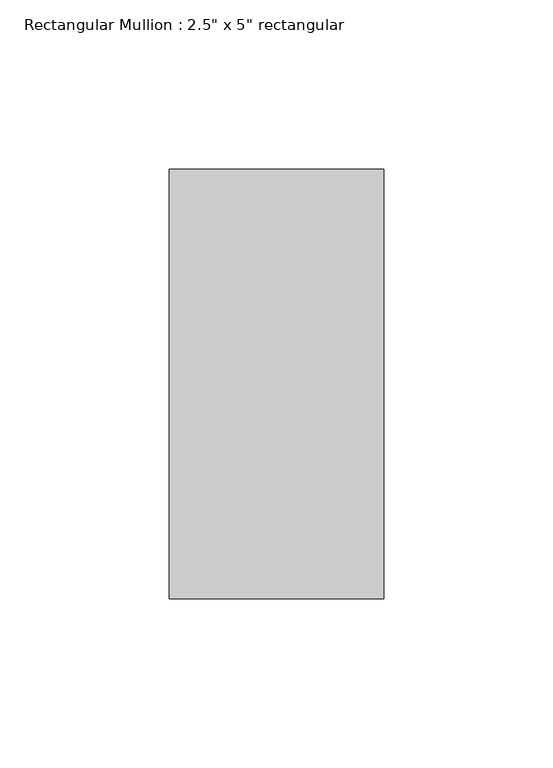
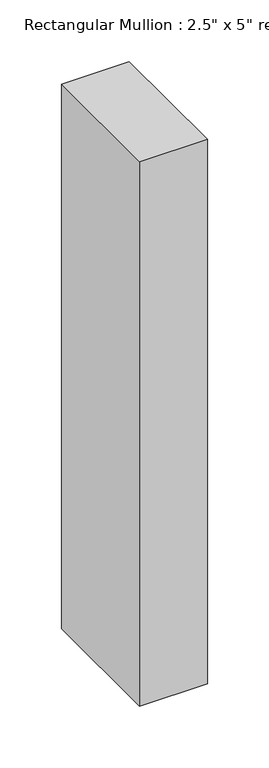
"""IFC4 building model written with IfcOpenShell, lengths in millimetres: member geometry."""

from ifc_helpers import new_model, si_unit, frame, origin, place, context, project, spatial, polyline, outline, extrude, source, transform, mapped, element, save


def member_81de2198(model_context):
    return source(origin(), model_context, "Body", "SweptSolid", [
        extrude(outline(polyline([(0.0, 63.5), (0.0, -63.5), (-63.5, -63.5), (-63.5, 63.5), (0.0, 63.5)])), frame((0.0, 0.0, -539.75), z_axis=(0.0, 0.0, 1.0), x_axis=(1.0, 0.0, 0.0)), (0.0, 0.0, 1.0), 539.75),
    ])


if __name__ == "__main__":
    model = new_model("IFC4")
    model_context = context("Model", 3, world=origin())
    ifc_project = project(units=[si_unit("LENGTHUNIT", "METRE", prefix="MILLI")], contexts=[model_context])
    site = spatial("IfcSite", under=ifc_project)
    building = spatial("IfcBuilding", under=site)
    placement = place(None, origin())
    member_shape = member_81de2198(model_context)
    element("IfcMember", 1, ObjectType="Rectangular Mullion : 2.5\" x 5\" rectangular", at=placement, inside=building, context=model_context, shape_type="MappedRepresentation", body=[
        mapped(member_shape, transform((0.0, 0.0, 0.0), x_axis=(1.0, 0.0, 0.0), y_axis=(0.0, 1.0, 0.0), z_axis=(0.0, 0.0, 1.0))),
    ])
    save(model, "model.ifc")

# Revit data of these elements
# Type "Rectangular Mullion : 2.5\" x 5\" rectangular"
#   built-in parameter 1007304 = 0.416667 (stored number, unit not read)
#   built-in parameter 1007301 = 0.104167 (stored number, unit not read)
#   built-in parameter 1007300 = 0.104167 (stored number, unit not read)
# Element 1 (IfcMember, "Rectangular Mullion : 2.5\" x 5\" rectangular")
#   Materials on its faces: "Aluminum"
# Materials
#   "Aluminum": class "Metal", colour RGB 247 247 247, transparency 0, Description = "Aluminum 6061", Cost = 0
